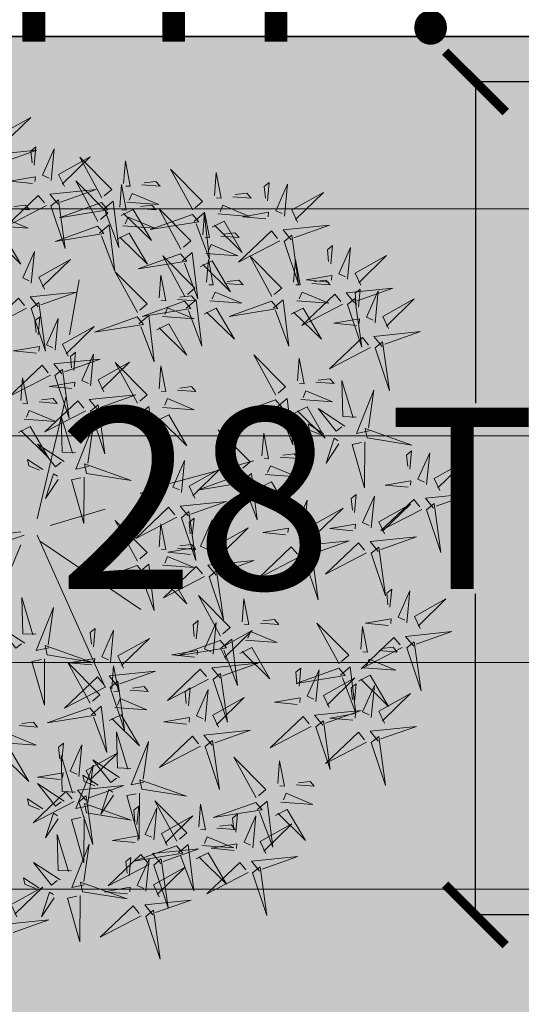
# Model space of a CAD drawing. Units: inches. Extents: x 1704 to 6393, y -157 to 1172.
# Tile 100 of 122: x 2577 to 2594, y 1001 to 1034. Entities that reach past the tile are written whole.
import ezdxf

# ---------------------------------------------------------------- set-up
doc = ezdxf.new("R2010")
doc.units = ezdxf.units.IN
doc.header["$MEASUREMENT"] = 0
for name, color, linetype, lineweight in [('A-ANNO-DIMS', 7, 'Continuous', 13), ('C-PROP', 7, 'Continuous', 35), ('L-DECK-PLNK-PATT', 250, 'Continuous', 13), ('L-shrub', 74, 'Continuous', 18), ('L-tree', 102, 'Continuous', 18)]:
    doc.layers.add(name, color=color, linetype=linetype, lineweight=lineweight)
doc.layers.add('L-DECK-PATT', color=35, linetype='Continuous', lineweight=13, true_color=0xa6725b)
doc.styles.get("Standard").update_dxf_attribs({"font": 'arial.ttf'})
doc.dimstyles.get("Standard").update_dxf_attribs({"dimtxt": 6, "dimasz": 2, "dimexe": 0.18, "dimexo": 0.0625, "dimgap": 0.09, "dimtad": 0, "dimtih": 1, "dimtoh": 1, "dimdec": 1, "dimzin": 0, "dimdsep": 46, "dimlunit": 3, "dimtxsty": 'Standard', "dimblk": 'ARCHTICK', "dimcen": 0.09, "dimadec": 0, "dimazin": 0, "dimtfac": 1, "dimtdec": 1, "dimtofl": 0, "dimtmove": 0, "dimatfit": 3, "dimfxl": 1, "dimtolj": 1, "dimtzin": 0, "dimarcsym": 0})

# ---------------------------------------------------------------- blocks, each defined once
blk = doc.blocks.new('bamboo')
at = {"layer": 'L-shrub'}
for p, q in [((43.5, 73), (278.2, 631.2)), ((-12.4, 39.5), (-247.1, 564.2)), ((-23.6, 61.9), (-370, 296.3)), ((32.3, 39.5), (390, 162.3)), ((43.5, 28.4), (300.5, 61.9)), ((-57.1, 6), (-247.1, -49.8)), ((-12.4, -16.3), (-113, -440.5)), ((-470.6, -139.1), (-761.2, -217.2)), ((-124.2, -652.6), (-157.7, -842.3))]:
    blk.add_line(p, q, dxfattribs=at)
for points in [[(-387.8, 1356.5), (-437.1, 1504.1), (-413.6, 1335.2), (-387.8, 1356.5)], [(-160.7, 1284.9), (-160, 1444.8), (-116.9, 1294.1), (-149.7, 1287.2)], [(-372, 1355), (-230.1, 1428.5), (-343.6, 1320.5), (-364.9, 1346.4)], [(79.4, 1419.1), (107.8, 1384.6), (-52.4, 1368.4), (70.8, 1412)], [(-756.4, 1206.5), (-805.8, 1354.1), (-782.2, 1185.2), (-756.4, 1206.5)], [(-412.1, 1350.9), (-383.7, 1316.4), (-543.9, 1300.2), (-420.7, 1343.8)], [(-415.1, 1179.2), (-464.4, 1326.8), (-440.9, 1157.9), (-415.1, 1179.2)], [(-70.9, 1292.4), (-27.7, 1358.5), (-55.4, 1272.9), (-68.6, 1281.5)], [(57.7, 1357.7), (77.5, 1316.1), (-31.5, 1255.3), (64.8, 1349.1)], [(-169.3, 1271.7), (-323, 1296.4), (-162.4, 1238.9), (-169.3, 1271.7)], [(-740.7, 1205), (-598.8, 1278.5), (-712.2, 1170.5), (-733.6, 1196.4)], [(-500.1, 1137.3), (-534, 1108.2), (-553.5, 1268), (-507.4, 1145.8)], [(-433.8, 1289.5), (-414, 1248), (-523, 1187.1), (-426.7, 1280.9)], [(-388.2, 1269.3), (-398.7, 1159.2), (-358.2, 1250.5), (-381.1, 1260.6)], [(-323.8, 1278.9), (-245.2, 1271.3), (-333.9, 1256.1), (-332.4, 1271.8)], [(-18, 1257.9), (35, 1223.4), (30.4, 1245.3), (-7, 1260.2)], [(-561.9, 1157.8), (-603.1, 1137.1), (-666.2, 1244.8), (-570.4, 1150.5)], [(-399.4, 1177.7), (-257.4, 1251.3), (-370.9, 1143.2), (-392.2, 1169.1)], [(-175.7, 1247.6), (-131.9, 1256.8), (-191.9, 1107.3), (-173.4, 1236.6)], [(-92.2, 1230.9), (0.4, 1170.5), (-61.7, 1248.7), (-81.3, 1233.2)], [(-780.7, 1200.9), (-752.3, 1166.4), (-912.5, 1150.2), (-789.3, 1193.8)], [(-329.8, 1216), (-335.8, 1153.1), (-318.6, 1167.3), (-322.7, 1207.4)], [(-131.4, 1199.8), (-85.3, 1198.1), (-81.9, 1073.4), (-120.4, 1202.1)], [(-439.4, 1173.7), (-411, 1139.2), (-571.2, 1122.9), (-448, 1166.6)], [(-494, 1113.1), (-347.5, 1165.5), (-515.9, 1138.5), (-494, 1113.1)], [(-174.3, 1012.2), (-173.7, 1172.1), (-130.6, 1021.4), (-163.4, 1014.5)], [(-802.5, 1139.6), (-782.6, 1098), (-891.6, 1037.1), (-795.3, 1130.9)], [(-692.4, 1128.9), (-613.8, 1121.3), (-702.5, 1106.1), (-701, 1121.8)], [(-835, 1007.8), (-876.2, 987.1), (-939.2, 1094.8), (-843.4, 1000.5)], [(-773.2, 987.3), (-807.1, 958.2), (-826.6, 1118), (-780.4, 995.8)], [(-756.8, 1119.3), (-767.3, 1009.2), (-726.8, 1100.5), (-749.7, 1110.6)], [(-581.3, 1111.7), (-691.5, 1120), (-599.4, 1081.4), (-589.8, 1104.4)], [(-461.1, 1112.3), (-441.3, 1070.7), (-550.3, 1009.8), (-454, 1103.7)], [(-495.2, 1097.3), (-418.8, 957), (-529.1, 1068.2), (-503.7, 1090.1)], [(-415.5, 1092), (-426, 981.9), (-385.5, 1073.2), (-408.4, 1083.4)], [(-365.5, 930.4), (-364.8, 1090.2), (-321.7, 939.6), (-354.5, 932.7)], [(-351.1, 1101.6), (-272.5, 1094), (-361.2, 1078.8), (-359.7, 1094.5)], [(-155.7, 961.1), (-205, 1108.7), (-181.5, 939.8), (-155.7, 961.1)], [(-698.4, 1066), (-704.4, 1003.1), (-687.2, 1017.3), (-691.3, 1057.4)], [(-633.3, 1052.3), (-696.3, 1057), (-681.8, 1040.1), (-641.8, 1045)], [(-570.3, 1047.5), (-576.3, 968.8), (-593.4, 1057.2), (-577.6, 1056)], [(-84.5, 1019.7), (-41.3, 1085.8), (-69, 1000.1), (-82.2, 1008.8)], [(-357.1, 1038.7), (-363.1, 975.8), (-345.9, 990), (-350, 1030.1)], [(-183, 999), (-336.7, 1023.7), (-176.1, 966.2), (-183, 999)], [(-140, 959.5), (2, 1033.1), (-111.5, 925), (-132.8, 950.9)], [(-767.1, 963.1), (-620.5, 1015.5), (-788.9, 988.5), (-767.1, 963.1)], [(-275.7, 937.9), (-232.5, 1004), (-260.1, 918.3), (-273.4, 927)], [(-31.6, 985.2), (21.3, 950.7), (16.7, 972.5), (-20.7, 987.5)], [(-854.3, 961.7), (-964.6, 970), (-872.5, 931.4), (-862.8, 954.4)], [(-180, 955.5), (-151.6, 921), (-311.8, 904.8), (-188.6, 948.4)], [(-189.3, 974.8), (-145.6, 984), (-205.5, 834.6), (-187, 963.9)], [(-105.9, 958.2), (-13.2, 897.8), (-75.4, 976), (-94.9, 960.5)], [(-768.3, 947.3), (-691.9, 807), (-802.2, 918.2), (-776.8, 940.1)], [(-374.1, 917.2), (-527.8, 941.9), (-367.2, 884.4), (-374.1, 917.2)], [(-145, 927.1), (-99, 925.4), (-95.6, 800.6), (-134.1, 929.4)], [(-1166, 756.5), (-1215.3, 904.1), (-1191.8, 735.2), (-1166, 756.5)], [(-906.4, 902.3), (-969.4, 907), (-954.8, 890.1), (-914.9, 895)], [(-843.4, 897.5), (-849.4, 818.8), (-866.4, 907.2), (-850.7, 906)], [(-592.6, 770.2), (-641.9, 917.8), (-618.4, 748.9), (-592.6, 770.2)], [(-380.5, 893), (-336.7, 902.2), (-396.6, 752.7), (-378.2, 882.1)], [(-297, 876.4), (-204.4, 816), (-266.5, 894.2), (-286.1, 878.7)], [(-201.7, 894.1), (-181.9, 852.5), (-290.9, 791.6), (-194.6, 885.5)], [(-222.7, 903.4), (-169.8, 868.9), (-174.4, 890.7), (-211.8, 905.7)], [(120.7, 803.3), (79.5, 782.6), (16.5, 890.3), (112.2, 796)], [(-156.1, 873.8), (-166.6, 763.7), (-126.1, 855), (-149, 865.2)], [(-91.7, 883.5), (-13.1, 875.8), (-101.8, 860.6), (-100.3, 876.4)], [(-1150.2, 755), (-1008.3, 828.6), (-1121.8, 720.5), (-1143.1, 746.4)], [(-974.8, 702), (-1024.2, 849.6), (-1000.7, 680.7), (-974.8, 702)], [(-576.8, 768.6), (-434.9, 842.2), (-548.4, 734.1), (-569.7, 760)], [(-336.2, 845.3), (-290.1, 843.6), (-286.7, 718.8), (-325.2, 847.6)], [(-97.7, 820.6), (-103.7, 757.7), (-86.5, 771.9), (-90.6, 811.9)], [(-199.8, 660.1), (-233.7, 630.9), (-253.2, 790.8), (-207, 668.5)], [(-1190.3, 750.9), (-1161.9, 716.5), (-1322.1, 700.2), (-1198.9, 743.8)], [(-959.1, 700.5), (-817.2, 774), (-930.7, 666), (-952, 691.8)], [(-616.9, 764.6), (-588.5, 730.1), (-748.7, 713.9), (-625.5, 757.5)], [(-261.6, 680.5), (-302.7, 659.9), (-365.8, 767.6), (-270, 673.2)], [(101.4, 757.2), (-8.9, 765.5), (83.2, 726.9), (92.9, 749.9)], [(-1212, 689.6), (-1192.2, 648), (-1301.2, 587.1), (-1204.9, 680.9)], [(-999.2, 696.4), (-970.7, 661.9), (-1131, 645.7), (-1007.8, 689.3)], [(-638.6, 703.2), (-618.8, 661.6), (-727.8, 600.7), (-631.5, 694.6)], [(-619.9, 538.4), (-669.2, 686), (-645.7, 517), (-619.9, 538.4)], [(-593, 682.9), (-603.5, 572.8), (-563, 664.1), (-585.9, 674.3)], [(-528.6, 692.6), (-450, 684.9), (-538.7, 669.7), (-537.2, 685.5)], [(-264.9, 565.6), (-314.3, 713.2), (-290.7, 544.3), (-264.9, 565.6)], [(-193.7, 635.8), (-47.1, 688.2), (-215.5, 661.2), (-193.7, 635.8)], [(49.3, 697.7), (-13.7, 702.5), (0.8, 685.5), (40.8, 690.4)], [(-1166.4, 669.3), (-1176.9, 559.2), (-1136.4, 650.5), (-1159.3, 660.7)], [(-1059.9, 523.7), (-1093.8, 494.6), (-1113.3, 654.4), (-1067.1, 532.2)], [(-1102, 678.9), (-1023.4, 671.3), (-1112.1, 656.1), (-1110.6, 671.8)], [(-1121.7, 544.2), (-1162.9, 523.5), (-1225.9, 631.2), (-1130.2, 536.9)], [(-1108, 616), (-1114, 553.1), (-1096.8, 567.3), (-1100.9, 607.4)], [(-1020.9, 635), (-1001.1, 593.4), (-1110, 532.6), (-1013.8, 626.4)], [(-975.2, 614.7), (-985.8, 504.7), (-945.3, 596), (-968.1, 606.1)], [(-910.8, 624.4), (-832.2, 616.8), (-921, 601.5), (-919.5, 617.3)], [(-534.6, 629.7), (-540.6, 566.8), (-523.4, 581), (-527.5, 621)], [(-280.9, 634.5), (-391.2, 642.7), (-299.1, 604.1), (-289.4, 627.2)], [(-249.2, 564.1), (-107.3, 637.7), (-220.7, 529.6), (-242.1, 555.5)], [(-194.9, 620.1), (-118.4, 479.7), (-228.8, 591), (-203.4, 612.8)], [(-37.8, 466.8), (-37.2, 626.6), (5.9, 476), (-26.9, 469.1)], [(-604.1, 536.8), (-462.2, 610.4), (-575.7, 502.3), (-597, 528.2)], [(-333, 575), (-396, 579.7), (-381.4, 562.8), (-341.5, 567.7)], [(-270, 570.3), (-276, 491.5), (-293, 579.9), (-277.2, 578.7)], [(-1288.8, 429.3), (-1338.2, 576.9), (-1314.7, 408), (-1288.8, 429.3)], [(-1053.8, 499.5), (-907.2, 551.9), (-1075.6, 524.9), (-1053.8, 499.5)], [(-916.9, 561.5), (-922.9, 498.6), (-905.6, 512.8), (-909.7, 552.9)], [(-650.3, 428.2), (-684.2, 399.1), (-703.7, 559), (-657.6, 436.7)], [(-289.2, 560), (-260.8, 525.6), (-421, 509.3), (-297.8, 552.9)], [(-712.1, 448.7), (-753.3, 428.1), (-816.4, 535.7), (-720.6, 441.4)], [(-644.2, 532.8), (-615.8, 498.3), (-776, 482), (-652.8, 525.7)], [(-1273.1, 427.7), (-1131.2, 501.3), (-1244.7, 393.3), (-1266, 419.1)], [(-1141, 498.1), (-1251.3, 506.4), (-1159.2, 467.8), (-1149.5, 490.8)], [(-1055, 483.7), (-978.6, 343.4), (-1088.9, 454.6), (-1063.5, 476.4)], [(-311, 498.7), (-291.1, 457.1), (-400.1, 396.2), (-303.9, 490)], [(-265.3, 478.4), (-275.8, 368.3), (-235.4, 459.6), (-258.2, 469.8)], [(-200.9, 488), (-122.3, 480.4), (-211, 465.2), (-209.5, 480.9)], [(-46.5, 453.6), (-200.1, 478.3), (-39.6, 420.8), (-46.5, 453.6)], [(-1193.1, 438.6), (-1256.1, 443.4), (-1241.5, 426.4), (-1201.6, 431.4)], [(-1130.1, 433.9), (-1136.1, 355.2), (-1153.1, 443.6), (-1137.4, 442.4)], [(-665.9, 471.4), (-646.1, 429.8), (-755.1, 368.9), (-658.8, 462.8)], [(-644.2, 404), (-497.6, 456.4), (-666, 429.4), (-644.2, 404)], [(-620.3, 451.1), (-630.8, 341), (-590.3, 432.3), (-613.2, 442.5)], [(-555.9, 460.7), (-477.3, 453.1), (-566, 437.9), (-564.5, 453.6)], [(-1313.2, 423.7), (-1284.7, 389.2), (-1445, 373), (-1321.8, 416.6)], [(-731.5, 402.7), (-841.7, 410.9), (-749.6, 372.3), (-739.9, 395.4)], [(-206.9, 425.1), (-212.9, 362.2), (-195.7, 376.4), (-199.8, 416.5)], [(-52.8, 429.4), (-9, 438.6), (-69, 289.1), (-50.5, 418.5)], [(30.7, 412.7), (123.3, 352.4), (61.2, 430.6), (41.6, 415)], [(-645.4, 388.3), (-569, 247.9), (-679.3, 359.1), (-653.9, 381)], [(-561.9, 397.8), (-567.9, 334.9), (-550.7, 349.1), (-554.8, 389.2)], [(-8.5, 381.7), (37.5, 380), (40.9, 255.2), (2.4, 384)], [(-1334.9, 362.3), (-1315.1, 320.7), (-1424, 259.8), (-1327.8, 353.7)], [(-1289.2, 342), (-1299.8, 231.9), (-1259.3, 323.3), (-1282.1, 333.4)], [(-1224.9, 351.7), (-1146.2, 344), (-1235, 328.8), (-1233.5, 344.6)], [(-783.5, 343.2), (-846.5, 347.9), (-832, 331), (-792, 335.9)], [(-720.5, 338.5), (-726.5, 259.7), (-743.5, 348.1), (-727.8, 346.9)], [(-606.2, 183.8), (-655.6, 331.4), (-632, 162.5), (-606.2, 183.8)], [(-1230.9, 288.8), (-1236.9, 225.9), (-1219.6, 240.1), (-1223.8, 280.1)], [(-425.4, 189.6), (-466.6, 169), (-529.7, 276.7), (-433.9, 182.4)], [(-363.6, 169.2), (-397.5, 140), (-417, 299.9), (-370.9, 177.6)], [(-1166, 102), (-1215.3, 249.6), (-1191.8, 80.7), (-1166, 102)], [(-933.9, 115.6), (-983.2, 263.3), (-959.7, 94.3), (-933.9, 115.6)], [(-590.5, 182.3), (-448.6, 255.9), (-562, 147.8), (-583.4, 173.7)], [(-1150.2, 100.5), (-1008.3, 174), (-1121.8, 66), (-1143.1, 91.9)], [(-918.2, 114.1), (-776.2, 187.7), (-889.7, 79.6), (-911, 105.5)], [(-630.5, 178.2), (-602.1, 143.7), (-762.3, 127.5), (-639.2, 171.1)], [(-357.5, 145), (-210.9, 197.3), (-379.3, 170.3), (-357.5, 145)], [(-444.7, 143.6), (-555, 151.8), (-462.9, 113.3), (-453.2, 136.3)], [(-958.2, 110.1), (-929.8, 75.6), (-1090, 59.3), (-966.8, 103)], [(-652.3, 116.9), (-632.5, 75.3), (-741.4, 14.4), (-645.2, 108.2)], [(-510.6, -20.7), (-560, 126.9), (-536.5, -42), (-510.6, -20.7)], [(-542.2, 106.2), (-463.6, 98.6), (-552.3, 83.4), (-550.8, 99.1)], [(-358.7, 129.2), (-282.3, -11.2), (-392.6, 100.1), (-367.2, 121.9)], [(-1357.1, -48), (-1406.5, 99.6), (-1382.9, -69.3), (-1357.1, -48)], [(-1190.3, 96.4), (-1161.9, 61.9), (-1322.1, 45.7), (-1198.9, 89.3)], [(-606.6, 96.6), (-617.1, -13.5), (-576.7, 77.8), (-599.5, 88)], [(-496.8, 84.1), (-559.8, 88.8), (-545.3, 71.9), (-505.3, 76.8)], [(-433.8, 79.4), (-439.8, 0.6), (-456.8, 89), (-441.1, 87.9)], [(-1212, 35.1), (-1192.2, -6.5), (-1301.2, -67.4), (-1204.9, 26.4)], [(-979.9, 48.7), (-960.1, 7.1), (-1069.1, -53.8), (-972.8, 40.1)], [(-869.9, 38), (-791.3, 30.4), (-880, 15.2), (-878.5, 30.9)], [(-548.2, 43.3), (-554.2, -19.6), (-537, -5.4), (-541.1, 34.7)], [(-494.9, -22.2), (-353, 51.3), (-466.5, -56.7), (-487.8, -30.9)], [(-1341.4, -49.5), (-1199.5, 24), (-1312.9, -84), (-1334.3, -58.1)], [(-1166.4, 14.8), (-1176.9, -95.3), (-1136.4, -4), (-1159.3, 6.1)], [(-1102, 24.4), (-1023.4, 16.8), (-1112.1, 1.6), (-1110.6, 17.3)], [(-934.3, 28.4), (-944.8, -81.7), (-904.3, 9.6), (-927.2, 19.8)], [(-875.9, -24.9), (-881.9, -87.8), (-864.7, -73.6), (-868.8, -33.5)], [(-718.6, -144.5), (-752.5, -173.6), (-772, -13.7), (-725.8, -136)], [(-535, -26.3), (-506.5, -60.8), (-666.8, -77), (-543.6, -33.4)], [(-174.3, -160.5), (-173.7, -0.6), (-130.6, -151.3), (-163.4, -158.2)], [(-1381.4, -53.6), (-1353, -88.1), (-1513.2, -104.3), (-1390.1, -60.7)], [(-1108, -38.5), (-1114, -101.4), (-1096.8, -87.2), (-1100.9, -47.1)], [(-780.4, -124), (-821.5, -144.7), (-884.6, -37), (-788.8, -131.3)], [(-556.7, -87.7), (-536.9, -129.3), (-645.8, -190.1), (-549.6, -96.3)], [(-446.7, -98.3), (-368, -105.9), (-456.8, -121.2), (-455.3, -105.4)], [(-84.5, -153), (-41.3, -86.9), (-69, -172.5), (-82.2, -163.9)], [(-1403.2, -114.9), (-1383.3, -156.5), (-1492.3, -217.4), (-1396.1, -123.6)], [(-1357.5, -135.2), (-1368, -245.3), (-1327.6, -154), (-1350.4, -143.9)], [(-1293.1, -125.6), (-1214.5, -133.2), (-1303.2, -148.4), (-1301.7, -132.7)], [(-1143.7, -283.2), (-1143, -123.3), (-1099.9, -274), (-1132.7, -280.9)], [(-712.5, -168.7), (-565.9, -116.3), (-734.3, -143.3), (-712.5, -168.7)], [(-511, -108), (-521.6, -218), (-481.1, -126.7), (-503.9, -116.6)], [(-799.7, -170.1), (-910, -161.8), (-817.9, -200.4), (-808.2, -177.3)], [(-452.7, -161.2), (-458.7, -224.1), (-441.4, -209.9), (-445.5, -169.8)], [(-183, -173.7), (-336.7, -149), (-176.1, -206.5), (-183, -173.7)], [(-1299.1, -188.5), (-1305.1, -251.4), (-1287.9, -237.2), (-1292, -197.1)], [(-713.7, -184.4), (-637.3, -324.8), (-747.6, -213.6), (-722.2, -191.7)], [(-189.3, -197.8), (-145.6, -188.6), (-205.5, -338.1), (-187, -208.8)], [(-105.9, -214.5), (-13.2, -274.9), (-75.4, -196.7), (-94.9, -212.2)], [(-31.6, -187.5), (21.3, -222), (16.7, -200.1), (-20.7, -185.2)], [(-1053.9, -275.7), (-1010.7, -209.6), (-1038.4, -295.3), (-1051.6, -286.6)], [(-851.8, -229.5), (-914.8, -224.8), (-900.2, -241.7), (-860.3, -236.8)], [(-788.8, -234.2), (-794.8, -313), (-811.8, -224.6), (-796, -225.8)], [(52.5, -314.9), (11.3, -335.6), (-51.8, -227.9), (44, -322.2)], [(-1152.3, -296.4), (-1306, -271.7), (-1145.4, -329.2), (-1152.3, -296.4)], [(-425.4, -355.8), (-466.6, -376.5), (-529.7, -268.8), (-433.9, -363.1)], [(-363.6, -376.3), (-397.5, -405.4), (-417, -245.5), (-370.9, -367.8)], [(-196.6, -388.9), (-246, -241.3), (-222.5, -410.2), (-196.6, -388.9)], [(-145, -245.6), (-99, -247.3), (-95.6, -372), (-134.1, -243.3)], [(-903.2, -383.1), (-944.4, -403.7), (-1007.5, -296), (-911.7, -390.3)], [(-841.4, -403.5), (-875.3, -432.7), (-894.8, -272.8), (-848.7, -395.1)], [(-1158.7, -320.6), (-1114.9, -311.4), (-1174.8, -460.8), (-1156.4, -331.5)], [(-1075.2, -337.2), (-982.6, -397.6), (-1044.7, -319.4), (-1064.3, -334.9)], [(-1000.9, -310.2), (-948, -344.7), (-952.6, -322.9), (-990, -307.9)], [(-180.9, -390.4), (-39, -316.9), (-152.5, -424.9), (-173.8, -399)], [(-1114.4, -368.3), (-1068.3, -370), (-1064.9, -494.8), (-1103.4, -366)], [(-357.5, -400.5), (-210.9, -348.1), (-379.3, -375.1), (-357.5, -400.5)], [(-73.8, -511.6), (-123.1, -364), (-99.6, -532.9), (-73.8, -511.6)], [(33.1, -361), (-77.2, -352.7), (14.9, -391.3), (24.6, -368.2)], [(-835.4, -427.8), (-688.8, -375.4), (-857.2, -402.4), (-835.4, -427.8)], [(-444.7, -401.9), (-555, -393.6), (-462.9, -432.2), (-453.2, -409.1)], [(-221, -394.5), (-192.5, -429), (-352.8, -445.2), (-229.6, -401.6)], [(-922.6, -429.1), (-1032.9, -420.9), (-940.7, -459.5), (-931.1, -436.4)], [(-358.7, -416.2), (-282.3, -556.6), (-392.6, -445.4), (-367.2, -423.5)], [(-19, -420.4), (-82, -415.7), (-67.4, -432.6), (-27.4, -427.7)], [(-58, -513.1), (83.9, -439.6), (-29.6, -547.6), (-50.9, -521.7)], [(44, -425.1), (38, -503.9), (21, -415.5), (36.8, -416.7)], [(-1179.6, -607.1), (-1229, -459.4), (-1205.5, -628.4), (-1179.6, -607.1)], [(-836.6, -443.5), (-760.1, -583.9), (-870.5, -472.6), (-845, -450.8)], [(-496.8, -461.3), (-559.8, -456.6), (-545.3, -473.5), (-505.3, -468.6)], [(-433.8, -466), (-439.8, -544.8), (-456.8, -456.4), (-441.1, -457.6)], [(-242.7, -455.8), (-222.9, -497.4), (-331.8, -558.3), (-235.6, -464.5)], [(-197, -476.1), (-207.5, -586.2), (-167.1, -494.9), (-189.9, -484.8)], [(-132.6, -466.5), (-54, -474.1), (-142.8, -489.3), (-141.3, -473.6)], [(-974.6, -488.6), (-1037.7, -483.9), (-1023.1, -500.8), (-983.1, -495.9)], [(-911.6, -493.3), (-917.6, -572.1), (-934.7, -483.7), (-918.9, -484.8)], [(-1163.9, -608.6), (-1022, -535), (-1135.5, -643.1), (-1156.8, -617.2)], [(-98.1, -517.2), (-69.7, -551.7), (-229.9, -567.9), (-106.7, -524.3)], [(-138.6, -529.4), (-144.7, -592.3), (-127.4, -578.1), (-131.5, -538)], [(-363.6, -689.9), (-397.5, -719), (-417, -559.2), (-370.9, -681.4)], [(-1084.1, -757), (-1133.4, -609.4), (-1109.9, -778.4), (-1084.1, -757)], [(-425.4, -669.4), (-466.6, -690.1), (-529.7, -582.4), (-433.9, -676.7)], [(-119.8, -578.6), (-100, -620.2), (-209, -681), (-112.7, -587.2)], [(-74.2, -598.9), (-84.7, -708.9), (-44.2, -617.6), (-67, -607.5)], [(8.2, -743.4), (-41.2, -595.8), (-17.7, -764.7), (8.2, -743.4)], [(-9.8, -589.2), (68.8, -596.8), (-19.9, -612), (-18.4, -596.3)], [(-1204, -612.6), (-1175.5, -647.1), (-1335.8, -663.4), (-1212.6, -619.7)], [(-889.6, -724), (-930.8, -744.6), (-993.8, -636.9), (-898.1, -731.2)], [(-827.8, -744.4), (-861.7, -773.6), (-881.2, -613.7), (-835.1, -736)], [(-589.2, -724), (-630.4, -744.6), (-693.5, -636.9), (-597.7, -731.2)], [(-527.4, -744.4), (-561.3, -773.6), (-580.8, -613.7), (-534.7, -736)], [(-1225.7, -674), (-1205.9, -715.6), (-1314.8, -776.5), (-1218.6, -682.6)], [(-357.5, -714.1), (-210.9, -661.7), (-379.3, -688.7), (-357.5, -714.1)], [(-15.8, -652.1), (-21.8, -715), (-4.6, -700.8), (-8.7, -660.7)], [(23.9, -744.9), (165.8, -671.4), (52.3, -779.4), (31, -753.6)], [(-1180, -694.3), (-1190.5, -804.4), (-1150.1, -713.1), (-1172.9, -702.9)], [(-1115.6, -684.7), (-1037, -692.3), (-1125.7, -707.5), (-1124.2, -691.8)], [(-1068.3, -758.6), (-926.4, -685), (-1039.9, -793.1), (-1061.2, -767.2)], [(-444.7, -715.5), (-555, -707.2), (-462.9, -745.8), (-453.2, -722.8)], [(-1121.6, -747.6), (-1127.7, -810.5), (-1110.4, -796.3), (-1114.5, -756.2)], [(-821.7, -768.6), (-675.1, -716.3), (-843.5, -743.3), (-821.7, -768.6)], [(-521.3, -768.6), (-374.8, -716.3), (-543.2, -743.3), (-521.3, -768.6)], [(-358.7, -729.9), (-282.3, -870.2), (-392.6, -759), (-367.2, -737.1)], [(-1108.4, -762.6), (-1079.9, -797.1), (-1240.2, -813.4), (-1117, -769.7)], [(-908.9, -770), (-1019.2, -761.8), (-927.1, -800.3), (-917.4, -777.3)], [(-608.6, -770), (-718.8, -761.8), (-626.7, -800.3), (-617.1, -777.3)], [(-513.8, -908.1), (-547.7, -937.2), (-567.2, -777.3), (-521, -899.6)], [(-496.8, -774.9), (-559.8, -770.2), (-545.3, -787.1), (-505.3, -782.2)], [(-433.8, -779.7), (-439.8, -858.4), (-456.8, -770), (-441.1, -771.2)], [(-16.2, -749), (12.3, -783.5), (-148, -799.7), (-24.8, -756.1)], [(-822.9, -784.4), (-746.5, -924.8), (-856.8, -813.5), (-831.4, -791.7)], [(-575.6, -887.6), (-616.8, -908.3), (-679.8, -800.6), (-584, -894.9)], [(-522.5, -784.4), (-446.1, -924.8), (-556.4, -813.5), (-531, -791.7)], [(-37.9, -810.4), (-18.1, -852), (-127, -912.8), (-30.8, -819)], [(-1130.1, -824), (-1110.3, -865.6), (-1219.3, -926.5), (-1123, -832.6)], [(-1084.5, -844.3), (-1095, -954.4), (-1054.5, -863.1), (-1077.3, -852.9)], [(-1020.1, -834.7), (-941.4, -842.3), (-1030.2, -857.5), (-1028.7, -841.8)], [(-961, -829.5), (-1024, -824.8), (-1009.5, -841.7), (-969.5, -836.8)], [(-898, -834.2), (-904, -913), (-921, -824.6), (-905.3, -825.7)], [(-865.6, -975.2), (-915, -827.6), (-891.5, -996.5), (-865.6, -975.2)], [(-660.6, -829.5), (-723.6, -824.8), (-709.1, -841.7), (-669.1, -836.8)], [(-597.6, -834.2), (-603.6, -913), (-620.7, -824.6), (-604.9, -825.7)], [(7.8, -830.7), (-2.8, -940.7), (37.7, -849.4), (14.9, -839.3)], [(-507.7, -932.3), (-361.1, -879.9), (-529.5, -906.9), (-507.7, -932.3)], [(-227.1, -1003.5), (-261, -1032.7), (-280.5, -872.8), (-234.3, -995)], [(-1026.1, -897.6), (-1032.1, -960.5), (-1014.9, -946.3), (-1019, -906.2)], [(-849.9, -976.7), (-708, -903.2), (-821.4, -1011.2), (-842.8, -985.4)], [(-554.7, -1044.4), (-588.6, -1073.6), (-608.1, -913.7), (-562, -1036)], [(-288.9, -983), (-330, -1003.7), (-393.1, -896), (-297.3, -990.3)], [(148, -983), (106.8, -1003.7), (43.8, -896), (139.5, -990.3)], [(-616.5, -1023.9), (-657.7, -1044.6), (-720.8, -936.9), (-625, -1031.2)], [(-594.9, -933.7), (-705.2, -925.4), (-613.1, -964), (-603.4, -940.9)], [(-508.9, -948), (-432.5, -1088.4), (-542.8, -977.2), (-517.4, -955.3)], [(-60.1, -1097.9), (-109.5, -950.3), (-85.9, -1119.2), (-60.1, -1097.9)], [(-889.9, -980.8), (-861.5, -1015.3), (-1021.7, -1031.5), (-898.6, -987.9)], [(-302.5, -1064.9), (-343.7, -1085.5), (-406.8, -977.8), (-311, -1072.1)], [(-240.7, -1085.3), (-274.6, -1114.5), (-294.1, -954.6), (-248, -1076.9)], [(-221, -1027.7), (-74.4, -975.4), (-242.8, -1002.3), (-221, -1027.7)], [(-647, -993.1), (-710, -988.4), (-695.4, -1005.3), (-655.5, -1000.4)], [(-584, -997.8), (-590, -1076.6), (-607, -988.2), (-591.3, -989.4)], [(-548.6, -1068.6), (-402.1, -1016.3), (-570.5, -1043.2), (-548.6, -1068.6)], [(-911.7, -1042.2), (-891.9, -1083.8), (-1000.8, -1144.6), (-904.6, -1050.8)], [(-801.6, -1052.8), (-723, -1060.4), (-811.7, -1075.7), (-810.2, -1059.9)], [(-308.2, -1029.1), (-418.5, -1020.8), (-326.4, -1059.4), (-316.7, -1036.4)], [(-222.2, -1043.5), (-145.8, -1183.9), (-256.1, -1072.6), (-230.7, -1050.8)], [(-44.4, -1099.5), (97.5, -1025.9), (-15.9, -1134), (-37.3, -1108.1)], [(128.7, -1029.1), (18.4, -1020.8), (110.5, -1059.4), (120.2, -1036.4)], [(-866, -1062.5), (-876.5, -1172.5), (-836.1, -1081.2), (-858.9, -1071.1)], [(-635.9, -1070), (-746.1, -1061.7), (-654, -1100.3), (-644.4, -1077.3)], [(-549.8, -1084.4), (-473.4, -1224.8), (-583.8, -1113.5), (-558.3, -1091.7)], [(-360.3, -1088.6), (-423.3, -1083.8), (-408.7, -1100.8), (-368.8, -1095.8)], [(-297.3, -1093.3), (-303.3, -1172), (-320.3, -1083.6), (-304.5, -1084.8)], [(-234.6, -1109.5), (-88.1, -1057.2), (-256.5, -1084.1), (-234.6, -1109.5)], [(76.6, -1088.6), (13.6, -1083.8), (28.1, -1100.8), (68.1, -1095.8)], [(-807.6, -1115.7), (-813.6, -1178.6), (-796.4, -1164.4), (-800.5, -1124.4)], [(-321.9, -1110.9), (-432.1, -1102.7), (-340, -1141.2), (-330.3, -1118.2)], [(-84.4, -1103.5), (-56, -1138), (-216.2, -1154.2), (-93.1, -1110.6)], [(-687.9, -1129.5), (-751, -1124.7), (-736.4, -1141.7), (-696.4, -1136.8)], [(-624.9, -1134.2), (-630.9, -1213), (-648, -1124.6), (-632.2, -1125.7)], [(-235.8, -1125.3), (-159.4, -1265.7), (-269.7, -1154.4), (-244.3, -1132.6)], [(-373.9, -1170.4), (-436.9, -1165.7), (-422.4, -1182.6), (-382.4, -1177.7)], [(-310.9, -1175.1), (-316.9, -1253.9), (-334, -1165.5), (-318.2, -1166.6)], [(-106.2, -1164.9), (-86.3, -1206.5), (-195.3, -1267.4), (-99.1, -1173.5)], [(-60.5, -1185.2), (-71, -1295.3), (-30.6, -1204), (-53.4, -1193.8)], [(3.9, -1175.6), (82.5, -1183.2), (-6.2, -1198.4), (-4.7, -1182.7)], [(120.3, -1239.9), (148.8, -1274.4), (-11.4, -1290.6), (111.7, -1247)], [(-2.1, -1238.5), (-8.1, -1301.4), (9.1, -1287.1), (5, -1247.1)], [(98.6, -1301.3), (118.4, -1342.9), (9.5, -1403.7), (105.7, -1309.9)]]:
    blk.add_lwpolyline(points, dxfattribs=at)
blk = doc.blocks.new('_ArchTick')
at = {"color": 0, "linetype": 'ByBlock', "const_width": 0.15}
blk.add_lwpolyline([(-0.5, -0.5), (0.5, 0.5)], dxfattribs=at)
blk = doc.blocks.new('*D88')
at = {"layer": 'A-ANNO-DIMS', "color": 0, "lineweight": -2, "transparency": 16777216}
for p, q in [((2596.639, 1031.77), (2596.639, 1036.222)), ((2625.54, 1031.77), (2625.54, 1036.222)), ((2596.639, 1036.042), (2594.639, 1036.042)), ((2625.54, 1036.042), (2596.639, 1036.042))]:
    blk.add_line(p, q, dxfattribs=at)
at = {"layer": 'Defpoints', "color": 0, "lineweight": -3, "transparency": 16777216}
for p in [(2596.639, 1036.042), (2596.639, 1031.707), (2625.54, 1031.707)]:
    blk.add_point(p, dxfattribs=at)
at = {"layer": 'A-ANNO-DIMS', "color": 0, "lineweight": -2, "transparency": 16777216, "xscale": 2, "yscale": 2, "zscale": 2, "rotation": 180}
blk.add_blockref('_ArchTick', (2596.639, 1036.042), dxfattribs=at)
at = {"layer": 'A-ANNO-DIMS', "color": 0, "lineweight": -2, "transparency": 16777216, "xscale": 2, "yscale": 2, "zscale": 2}
blk.add_blockref('_ArchTick', (2625.54, 1036.042), dxfattribs=at)
at = {"layer": 'A-ANNO-DIMS', "color": 0, "transparency": 16777216, "insert": (2560.165, 1036.042), "char_height": 6, "attachment_point": 5}
blk.add_mtext('\\A1;SHRUB A 29 TYP.', dxfattribs=at)
blk = doc.blocks.new('*D89')
at = {"layer": 'A-ANNO-DIMS', "color": 0, "lineweight": -2, "transparency": 16777216}
for p, q in [((2596.576, 1031.707), (2592.123, 1031.707)), ((2592.303, 1031.707), (2592.303, 1021.085)), ((2592.303, 1004.156), (2592.303, 1014.778)), ((2596.576, 1004.156), (2592.123, 1004.156))]:
    blk.add_line(p, q, dxfattribs=at)
at = {"layer": 'Defpoints', "color": 0, "lineweight": -3, "transparency": 16777216}
for p in [(2596.639, 1031.707), (2592.303, 1004.156), (2596.639, 1004.156)]:
    blk.add_point(p, dxfattribs=at)
at = {"layer": 'A-ANNO-DIMS', "color": 0, "lineweight": -2, "transparency": 16777216, "xscale": 2, "yscale": 2, "zscale": 2}
for p, rotation in [((2592.303, 1031.707), 90), ((2592.303, 1004.156), 270)]:
    blk.add_blockref('_ArchTick', p, dxfattribs=dict(at, rotation=rotation))
at = {"layer": 'A-ANNO-DIMS', "color": 0, "transparency": 16777216, "insert": (2592.303, 1017.931), "char_height": 6, "attachment_point": 5}
blk.add_mtext('\\A1;28 TYP.', dxfattribs=at)
blk = doc.blocks.new('*D92')
at = {"layer": 'A-ANNO-DIMS', "color": 0, "lineweight": -2, "transparency": 16777216}
for p, q in [((2073.349, 895.275), (2073.349, 1105.287)), ((2605.349, 895.275), (2605.349, 1105.287)), ((2073.349, 1105.107), (2332.661, 1105.107)), ((2605.349, 1105.107), (2346.036, 1105.107))]:
    blk.add_line(p, q, dxfattribs=at)
at = {"layer": 'Defpoints', "color": 0, "lineweight": -3, "transparency": 16777216}
for p in [(2605.349, 1105.107), (2073.349, 895.213), (2605.349, 895.213)]:
    blk.add_point(p, dxfattribs=at)
at = {"layer": 'A-ANNO-DIMS', "color": 0, "lineweight": -2, "transparency": 16777216, "xscale": 2, "yscale": 2, "zscale": 2, "rotation": 180}
blk.add_blockref('_ArchTick', (2073.349, 1105.107), dxfattribs=at)
at = {"layer": 'A-ANNO-DIMS', "color": 0, "lineweight": -2, "transparency": 16777216, "xscale": 2, "yscale": 2, "zscale": 2}
blk.add_blockref('_ArchTick', (2605.349, 1105.107), dxfattribs=at)
at = {"layer": 'A-ANNO-DIMS', "color": 0, "transparency": 16777216, "insert": (2339.349, 1105.107), "char_height": 6, "attachment_point": 5}
blk.add_mtext('\\A1;532', dxfattribs=at)
blk = doc.blocks.new('*D103')
at = {"layer": 'A-ANNO-DIMS', "color": 0, "lineweight": -2, "transparency": 16777216}
for p, q in [((2551.349, 711.275), (2551.349, 1105.287)), ((2597.349, 711.275), (2597.349, 1105.287)), ((2551.349, 1105.107), (2569.842, 1105.107)), ((2597.349, 1105.107), (2578.855, 1105.107))]:
    blk.add_line(p, q, dxfattribs=at)
at = {"layer": 'Defpoints', "color": 0, "lineweight": -3, "transparency": 16777216}
for p in [(2597.349, 1105.107), (2551.349, 711.213), (2597.349, 711.213)]:
    blk.add_point(p, dxfattribs=at)
at = {"layer": 'A-ANNO-DIMS', "color": 0, "lineweight": -2, "transparency": 16777216, "xscale": 2, "yscale": 2, "zscale": 2, "rotation": 180}
blk.add_blockref('_ArchTick', (2551.349, 1105.107), dxfattribs=at)
at = {"layer": 'A-ANNO-DIMS', "color": 0, "lineweight": -2, "transparency": 16777216, "xscale": 2, "yscale": 2, "zscale": 2}
blk.add_blockref('_ArchTick', (2597.349, 1105.107), dxfattribs=at)
at = {"layer": 'A-ANNO-DIMS', "color": 0, "transparency": 16777216, "insert": (2574.349, 1105.107), "char_height": 6, "attachment_point": 5}
blk.add_mtext('\\A1;46', dxfattribs=at)

msp = doc.modelspace()

# ---------------------------------------------------------------- hatches: boundary and pattern name
at = {"layer": 'L-DECK-PATT', "transparency": 33554544}
h = msp.add_hatch(color=256, dxfattribs=at)
h.dxf.hatch_style = 1
h.paths.add_polyline_path([(2329.589, 1033.213), (2065.589, 1033.213), (2065.589, 895.213), (2167.349, 895.213), (2263.349, 895.213), (2263.349, 903.213), (2273.349, 903.213), (2273.349, 895.213), (2329.589, 895.213)])
h.paths.add_polyline_path([(2664.349, 1033.213), (2333.589, 1033.213), (2333.589, 895.213), (2465.349, 895.213), (2469.181, 895.213), (2470.482, 895.213), (2508.215, 895.213), (2509.516, 895.213), (2513.349, 895.213), (2533.349, 895.213), (2581.349, 895.213), (2605.349, 895.213), (2664.349, 895.213)])
h.paths.add_polyline_path([(2333.589, 1033.213), (2329.589, 1033.213), (2329.589, 895.213), (2333.589, 895.213)])
at = {"layer": 'L-DECK-PLNK-PATT'}
h = msp.add_hatch(dxfattribs=at)
h.set_pattern_fill('LINE', color=256, scale=60)
h.paths.add_polyline_path([(2329.589, 1033.213), (2065.589, 1033.213), (2065.589, 895.213), (2167.349, 895.213), (2263.349, 895.213), (2263.349, 903.213), (2273.349, 903.213), (2273.349, 895.213), (2329.589, 895.213)])
h.paths.add_polyline_path([(2664.349, 1033.213), (2333.589, 1033.213), (2333.589, 895.213), (2465.349, 895.213), (2469.181, 895.213), (2470.482, 895.213), (2508.215, 895.213), (2509.516, 895.213), (2513.349, 895.213), (2533.349, 895.213), (2581.349, 895.213), (2605.349, 895.213), (2664.349, 895.213)])
h.paths.add_polyline_path([(2333.589, 1033.213), (2329.589, 1033.213), (2329.589, 895.213), (2333.589, 895.213)])

# ---------------------------------------------------------------- linework, layer by layer
at = {"layer": 'C-PROP'}
msp.add_line((2723.349, 1033.213), (1898.349, 1033.213), dxfattribs=at)

# ---------------------------------------------------------------- block references
at = {"layer": 'L-tree', "xscale": 0.0095734028514679, "yscale": 0.0095734028514679, "zscale": 0.0095734028514679, "rotation": 180}
msp.add_blockref('bamboo', (2577.692, 1017.096), dxfattribs=at)

# ---------------------------------------------------------------- dimensions: what is measured, and where the dimension line sits
at = {"layer": 'A-ANNO-DIMS'}
for base, p1, p2, picture, middle in [((2605.349, 1105.107), (2073.349, 895.213), (2605.349, 895.213), '*D92', (2339.349, 1105.107)), ((2597.349, 1105.107), (2551.349, 711.213), (2597.349, 711.213), '*D103', (2574.349, 1105.107))]:
    dim = msp.add_linear_dim(base=base, p1=p1, p2=p2, dimstyle='Standard', override={"dimdec": 0, "dimlfac": 1, "dimrnd": 0, "dimzin": 0, "dimdsep": 46, "dimlunit": 2}, dxfattribs=at)
    dim.commit()
    dim.dimension.update_dxf_attribs({"geometry": picture, "text_midpoint": middle})
for base, p1, p2, angle, text, picture, middle in [((2596.639, 1036.042), (2625.54, 1031.707), (2596.639, 1031.707), 180, 'SHRUB A <> TYP.', '*D88', (2560.165, 1036.042)), ((2592.303, 1004.156), (2596.639, 1031.707), (2596.639, 1004.156), 270, '<> TYP.', '*D89', (2592.303, 1017.931))]:
    dim = msp.add_linear_dim(base=base, p1=p1, p2=p2, angle=angle, text=text, dimstyle='Standard', override={"dimdec": 0, "dimlfac": 1, "dimrnd": 0, "dimzin": 0, "dimdsep": 46, "dimlunit": 2}, dxfattribs=at)
    dim.commit()
    dim.dimension.update_dxf_attribs({"geometry": picture, "text_midpoint": middle})

doc.saveas('drawing.dxf')
